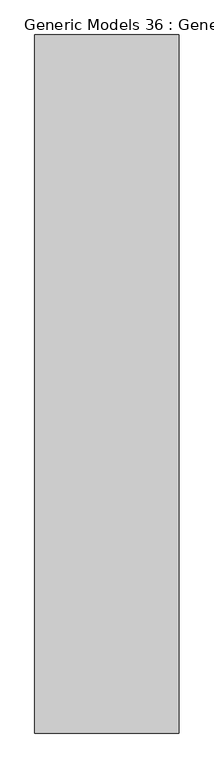
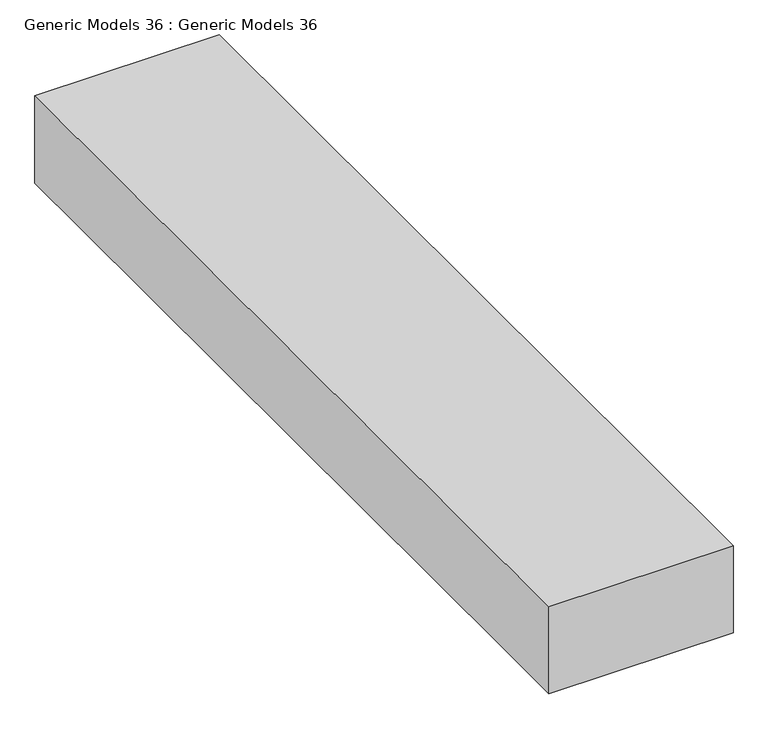
"""IFC4 building model written with IfcOpenShell, lengths in millimetres: proxy geometry, Generic Models 36 : Generic Models 36."""

from ifc_helpers import new_model, si_unit, frame, origin, place, context, project, spatial, polyline, outline, extrude, source, transform, mapped, element, save


def generic_models_36_generic_models_36_9c63594f(model_context):
    return source(origin(), model_context, "Body", "SweptSolid", [
        extrude(outline(polyline([(7518.1309003, 17459.2), (7391.1309003, 17459.2), (7391.1309003, 17611.6), (8864.3309003, 17611.6), (8864.3309003, 17459.2), (8737.3309003, 17459.2), (7518.1309003, 17459.2)])), frame((-6737.3887202, 0.0, 0.0), z_axis=(1.0, 0.0, 0.0), x_axis=(0.0, 1.0, 0.0)), (0.0, 0.0, 1.0), 304.8),
    ])


if __name__ == "__main__":
    model = new_model("IFC4")
    model_context = context("Model", 3, world=origin())
    ifc_project = project(units=[si_unit("LENGTHUNIT", "METRE", prefix="MILLI")], contexts=[model_context])
    site = spatial("IfcSite", under=ifc_project)
    building = spatial("IfcBuilding", under=site)
    placement = place(None, origin())
    generic_models_36_generic_models_36_shape = generic_models_36_generic_models_36_9c63594f(model_context)
    element("IfcBuildingElementProxy", 1, Name="Generic Models 36 : Generic Models 36", ObjectType="Generic Models 36 : Generic Models 36", at=placement, inside=building, context=model_context, shape_type="MappedRepresentation", body=[
        mapped(generic_models_36_generic_models_36_shape, transform((0.0, 0.0, 0.0), x_axis=(1.0, 0.0, 0.0), y_axis=(0.0, 1.0, 0.0), z_axis=(0.0, 0.0, 1.0))),
    ])
    save(model, "model.ifc")

# Revit data of these elements
# Element 1 (IfcBuildingElementProxy, "Generic Models 36 : Generic Models 36")
#   Materials on its faces: "white"
# Materials
#   "white": class "Generic", colour RGB 120 120 120, transparency 0, Cost = 0
